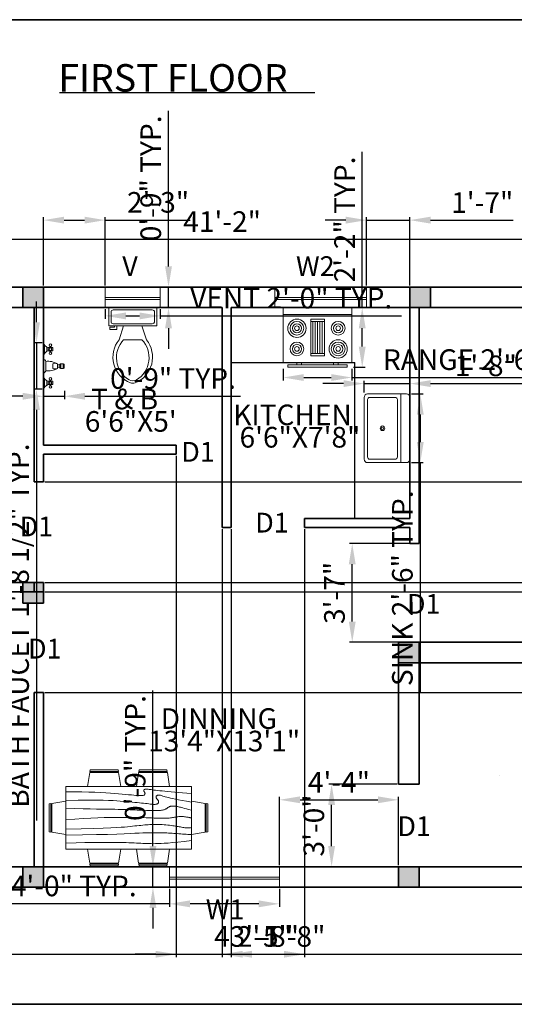
# Model space of a CAD drawing. Units: inches. Extents: x -281 to 2337, y 1647 to 2113.
# Tile 5 of 6: x 1906 to 2121, y 1674 to 2103. Entities that reach past the tile are written whole.
import ezdxf

# ---------------------------------------------------------------- set-up
doc = ezdxf.new("R2010")
doc.units = ezdxf.units.IN
for name, color, linetype, lineweight in [('A-ANNO-DIMS', 242, 'Continuous', 18), ('A-ANNO-IDEN', 11, 'Continuous', 18), ('A-ANNO-TEXT', 7, 'Continuous', 25), ('A-ANNO-TTLB', 7, 'Continuous', 35), ('A-AREA-IDEN', 7, 'Continuous', 18), ('A-COLS', 1, 'Continuous', 35), ('A-EQPM', 8, 'Continuous', 18), ('A-FLOR-CASE', 8, 'Continuous', 25), ('A-FLOR-FIXT', 8, 'Continuous', 18), ('A-FLOR-STRS', 7, 'Continuous', 18), ('A-FURN', 8, 'Continuous', 18), ('A-GLAZ', 3, 'Continuous', 18), ('A-WALL', 7, 'Continuous', 35)]:
    doc.layers.add(name, color=color, linetype=linetype, lineweight=lineweight)
doc.styles.get("Standard").update_dxf_attribs({"font": 'arial.ttf'})
doc.dimstyles.new('ISO-25', dxfattribs={"dimtxt": 9, "dimasz": 9, "dimexe": 1.25, "dimexo": 0.625, "dimgap": 2, "dimtad": 1, "dimdec": 1, "dimlunit": 4, "dimtxsty": 'Standard', "dimcen": 2.5, "dimadec": 0, "dimazin": 0, "dimtfac": 1, "dimtdec": 1, "dimtmove": 0, "dimatfit": 3, "dimfxl": 1, "dimarcsym": 0})

# ---------------------------------------------------------------- blocks, each defined once
blk = doc.blocks.new('Range-Oven - 30 in top')
for p, q in [((0, -3), (30, -3)), ((12, -6), (18, -6)), ((13, -20), (13, -6)), ((14, -6), (14, -20)), ((15, -20), (15, -6)), ((16, -6), (16, -20)), ((17, -20), (17, -6)), ((18, -20), (12, -20)), ((6, -24), (6, -25)), ((8, -25), (8, -24)), ((22, -25), (22, -24)), ((24, -24), (24, -25))]:
    blk.add_line(p, q)
for points in [[(0, -24), (0, 0), (30, 0), (30, -24)], [(12, -21), (12, -5), (18, -5), (18, -21)], [(2, -26), (2, -25), (28, -25), (28, -26)]]:
    blk.add_lwpolyline(points, close=True)
for centre, radius in [((6, -9), 4), ((6, -9), 3), ((6, -9), 2), ((6, -9), 1), ((24, -9), 3), ((24, -9), 2), ((24, -9), 1), ((6, -18), 3), ((6, -18), 2), ((6, -18), 1), ((24, -18), 4), ((24, -18), 3), ((24, -18), 2), ((24, -18), 1)]:
    blk.add_circle(centre, radius)
blk = doc.blocks.new('Sink-single - 30 in top')
blk.add_line((-15, -3.999996), (15, -3.999996))
for points in [[(-13.5, 0), (13.5, 0)], [(-15, -18.499996), (-15, -1.5)], [(15, -1.5), (15, -18.499996)], [(-13.5, -17.499996), (-13.5, -6.499996)], [(-12.5, -5.499996), (12.5, -5.499996)], [(13.5, -6.499996), (13.5, -17.499996)], [(13.5, -19.999996), (-13.5, -19.999996)], [(12.5, -18.499996), (-12.5, -18.499996)]]:
    blk.add_lwpolyline(points)
for radius in [1, 0.5]:
    blk.add_circle((0, -11.999996), radius)
for centre, radius, start, end in [((-13.5, -1.5), 1.5, 90, 180), ((13.5, -1.5), 1.5, 0, 90), ((-12.5, -6.499996), 1, 90, 180), ((12.5, -6.499996), 1, 0, 90), ((-13.5, -18.499996), 1.5, 180, 270), ((-12.5, -17.499996), 1, 180, 270), ((12.5, -17.499996), 1, 270, 0), ((13.5, -18.499996), 1.5, 270, 0)]:
    blk.add_arc(centre, radius, start, end)
blk = doc.blocks.new('Toilet - top')
for p, q in [((9.5, -6), (9.5, -2)), ((-10, -8.5), (-8, -8.5)), ((-10, -9.5), (-10, -8.5)), ((-8, -8.5), (-8, -8)), ((-7, -8), (-7, -9.5)), ((-4, -8), (-6, -14)), ((4, -8), (6, -14)), ((-7, -9.5), (-10, -9.5)), ((4, -14), (-4, -14))]:
    blk.add_line(p, q)
blk.add_lwpolyline([(10.5, -8), (10.5, 0), (-10.5, 0), (-10.5, -8)], close=True)
for points in [[(-9.5, -2), (-9.5, -6)], [(8.5, -1), (-8.5, -1)], [(-8.5, -7), (8.5, -7)]]:
    blk.add_lwpolyline(points)
for centre, radius, start, end in [((-8.62, -1.88), 0.884, 81.8699, 188.1301), ((8.62, -1.88), 0.884, 351.8699, 98.1301), ((-8.62, -6.12), 0.884, 171.8699, 278.1301), ((8.62, -6.12), 0.884, 261.8699, 8.1301), ((3.52, -21.58), 12.17, 141.4691, 247.9714), ((4.2, -21.82), 11.33, 136.3677, 238.9468), ((-3.52, -21.58), 12.17, 292.0284, 38.5307), ((-4.2, -21.82), 11.33, 301.053, 43.6321), ((0, -27.88), 4, 245.7318, 294.2682), ((0, -29), 4, 254.8605, 285.1395)]:
    blk.add_arc(centre, radius, start, end)
blk = doc.blocks.new('Faucet - Bathroom front')
for p, q in [((-0.5, 4.25), (0.5, 4.25)), ((0.5, 3.75), (-0.5, 3.75)), ((-0.5, 3), (0.5, 3)), ((-0.25, 3), (-0.25, 3.5)), ((0.25, 3.5), (0.25, 3)), ((-5, 0), (-2.25, 0)), ((-4.5087, 0.25), (-2.7408, 0.25)), ((-4, 1.625), (-4.25, 1.625)), ((-4, 1.375), (-4.25, 1.375)), ((-3.1442, 0.75), (-4.0979, 0.75)), ((-3.25, 1.625), (-3, 1.625)), ((-3.25, 1.375), (-3, 1.375)), ((-1.5, 0), (1.5, 0)), ((-1, 0.5), (1, 0.5)), ((0.5, 2), (-0.5, 2)), ((2.25, 0), (5, 0)), ((2.7413, 0.25), (4.5092, 0.25)), ((3.25, 1.625), (3, 1.625)), ((3.25, 1.375), (3, 1.375)), ((4.1058, 0.75), (3.1521, 0.75)), ((4, 1.625), (4.25, 1.625)), ((4, 1.375), (4.25, 1.375))]:
    blk.add_line(p, q)
for points in [[(-0.5, 3.75), (-0.5, 4.25)], [(-0.25, 4.5), (0.25, 4.5)], [(0.5, 4.25), (0.5, 3.75)], [(0.25, 3.5), (-0.25, 3.5)]]:
    blk.add_lwpolyline(points)
for points in [[(-4, 1), (-4, 2), (-3.25, 2), (-3.25, 1)], [(3.25, 1), (3.25, 2), (4, 2), (4, 1)]]:
    blk.add_lwpolyline(points, close=True)
for centre in [(-4.5, 1.5), (-3.625, 1.5), (-2.75, 1.5), (2.75, 1.5), (3.625, 1.5), (4.5, 1.5)]:
    blk.add_circle(centre, 0.2795)
for centre, radius, start, end in [((-0.2575, 4.2575), 0.2426, 88.22243, 181.7776), ((0.2575, 4.2575), 0.2426, 358.2224, 91.77757), ((3, 1), 4.0311, 150.2551, 187.125), ((0.6413, 2.5), 1.246, 156.3417, 203.6583), ((-0.2575, 3.7425), 0.2426, 178.2224, 271.7776), ((0.2575, 3.7425), 0.2426, 268.2224, 1.777565), ((-3, 1), 4.0311, 352.875, 29.74488), ((-0.6413, 2.5), 1.246, 336.3417, 23.65835), ((-5.375, 1.375), 1.4252, 285.2551, 344.7449), ((-1.875, 1.375), 1.4252, 195.2551, 254.7449), ((-0.7962, -0.2038), 0.7327, 106.1502, 163.8498), ((0.7962, -0.2038), 0.7327, 16.1502, 73.84979), ((1.875, 1.375), 1.4252, 285.2551, 344.7449), ((5.375, 1.375), 1.4252, 195.2551, 254.7449)]:
    blk.add_arc(centre, radius, start, end)
blk = doc.blocks.new('Dining Set - 36 x 72 in.')
for p, q in [((-22.2343, 26.00059), (-23.4847, 17.99762)), ((-22.2304, 26), (-5.7608, 26)), ((-22, 27.5), (-22.1562, 26.50042)), ((-5.8416, 26.5), (-22.1534, 26.5)), ((-22, 27.5), (-6, 27.5)), ((-5.8437, 26.49966), (-6, 27.5)), ((-4.5152, 17.99762), (-5.7655, 25.99926)), ((5.7657, 26.00059), (4.5153, 17.99762)), ((5.7696, 26), (22.2392, 26)), ((6, 27.5), (5.8438, 26.50042)), ((22.1584, 26.5), (5.8466, 26.5)), ((6, 27.5), (22, 27.5)), ((22.1563, 26.49966), (22, 27.5)), ((23.4848, 17.99762), (22.2345, 25.99926)), ((36, 18), (-36, 18)), ((-36, 18), (-36, -18)), ((36, -18), (36, 18)), ((-45.5, 8), (-44.5004, 8.15617)), ((-45.5, 8), (-45.5, -8)), ((-44.5, -8.15843), (-44.5, 8.15338)), ((-44.0006, 8.23428), (-35.9976, 9.48474)), ((-44, 8.23041), (-44, -8.23915)), ((44.0006, 8.23428), (35.9976, 9.48474)), ((44, 8.23041), (44, -8.23915)), ((44.5, -8.15843), (44.5, 8.15338)), ((45.5, 8), (44.5005, 8.15617)), ((45.5, 8), (45.5, -8)), ((-44.4997, -8.15631), (-45.5, -8)), ((-35.9976, -9.48476), (-43.9993, -8.2345)), ((35.9976, -9.48476), (43.9993, -8.2345)), ((44.4997, -8.15631), (45.5, -8)), ((-36, -18), (36, -18)), ((-22.2343, -26.0006), (-23.4847, -17.99762)), ((-4.5152, -17.99762), (-5.7655, -25.99928)), ((5.7657, -26.0006), (4.5153, -17.99762)), ((23.4848, -17.99762), (22.2345, -25.99928)), ((-22.2304, -26), (-5.7608, -26)), ((-22, -27.5), (-22.1562, -26.50044)), ((-5.8416, -26.5), (-22.1534, -26.5)), ((-22, -27.5), (-6, -27.5)), ((-5.8437, -26.49967), (-6, -27.5)), ((5.7696, -26), (22.2392, -26)), ((6, -27.5), (5.8438, -26.50044)), ((22.1584, -26.5), (5.8466, -26.5)), ((6, -27.5), (22, -27.5)), ((22.1563, -26.49967), (22, -27.5))]:
    blk.add_line(p, q)
for points in [[(-36, 15), (-31.1772, 14.97754), (-26.8079, 14.91406), (-22.8538, 14.81543), (-19.276, 14.6875), (-16.0362, 14.53613), (-13.0957, 14.36718), (-10.4159, 14.18652), (-7.9583, 14), (-5.6904, 13.81315), (-3.6035, 13.63021), (-1.6954, 13.45508), (0.0365, 13.29166), (1.5945, 13.14388), (2.9811, 13.01562), (4.1988, 12.9108), (5.25, 12.83333), (6.1393, 12.78613), (6.8802, 12.76823), (7.4883, 12.77767), (7.9792, 12.8125), (8.3685, 12.87077), (8.6719, 12.95052), (8.9049, 13.0498), (9.0833, 13.16666), (9.2205, 13.29899), (9.3216, 13.44401), (9.3895, 13.59879), (9.4271, 13.76041), (9.4373, 13.92594), (9.4232, 14.09245), (9.3875, 14.257), (9.3333, 14.41666), (9.2638, 14.56917), (9.1836, 14.71484), (9.0975, 14.85465), (9.0104, 14.98958), (8.9272, 15.1206), (8.8529, 15.2487), (8.7922, 15.37483), (8.75, 15.5), (8.7305, 15.62467), (8.7344, 15.74739), (8.7617, 15.86621), (8.8125, 15.97916), (8.8867, 16.08431), (8.9844, 16.17968), (9.1055, 16.26334), (9.25, 16.33333), (9.4189, 16.38802), (9.6172, 16.42708), (9.8506, 16.45052), (10.125, 16.45833), (10.4463, 16.45052), (10.8203, 16.42708), (11.2529, 16.38802), (11.75, 16.33333), (12.3184, 16.26318), (12.9694, 16.17838), (13.7151, 16.07991), (14.5677, 15.96875), (15.5395, 15.84586), (16.6426, 15.71224), (17.8893, 15.56884), (19.2917, 15.41666), (20.859, 15.25667), (22.5879, 15.08984), (24.4721, 14.91715), (26.5052, 14.73958), (28.6809, 14.5581), (30.9929, 14.3737), (33.4347, 14.18733), (36, 14)], [(-36, 10), (-28.9766, 10.14274), (-23.1725, 10.20442), (-18.4241, 10.19775), (-14.5677, 10.13541), (-11.4399, 10.03011), (-8.877, 9.89453), (-6.7154, 9.74137), (-4.7917, 9.58333), (-2.9698, 9.43082), (-1.2246, 9.28515), (0.4415, 9.14534), (2.026, 9.01041), (3.5266, 8.87939), (4.9408, 8.7513), (6.266, 8.62516), (7.5, 8.5), (8.6411, 8.37549), (9.6914, 8.2539), (10.6538, 8.13818), (11.5312, 8.03125), (12.3267, 7.93603), (13.043, 7.85547), (13.6831, 7.79248), (14.25, 7.75), (14.7471, 7.7303), (15.1797, 7.73307), (15.5537, 7.75732), (15.875, 7.80208), (16.1494, 7.86637), (16.3828, 7.94922), (16.5811, 8.04964), (16.75, 8.16666), (16.8944, 8.29915), (17.0143, 8.44531), (17.1089, 8.60319), (17.1771, 8.77083), (17.218, 8.94629), (17.2305, 9.1276), (17.2137, 9.31282), (17.1667, 9.5), (17.0895, 9.6875), (16.987, 9.875), (16.8649, 10.0625), (16.7292, 10.25), (16.5856, 10.4375), (16.4401, 10.625), (16.2985, 10.8125), (16.1667, 11), (16.05, 11.18733), (15.9518, 11.3737), (15.8752, 11.5581), (15.8229, 11.73958), (15.798, 11.91715), (15.8034, 12.08984), (15.842, 12.25667), (15.9167, 12.41666), (16.0295, 12.56836), (16.1784, 12.70833), (16.3605, 12.83268), (16.5729, 12.9375), (16.8127, 13.01888), (17.0768, 13.07291), (17.3625, 13.0957), (17.6667, 13.08333), (17.9894, 13.03312), (18.3418, 12.94726), (18.7382, 12.82918), (19.1927, 12.68229), (19.7195, 12.51001), (20.3327, 12.31575), (21.0465, 12.10294), (21.875, 11.875), (22.8357, 11.63354), (23.959, 11.37304), (25.2786, 11.08618), (26.8282, 10.76562), (28.6414, 10.40405), (30.752, 9.99414), (33.1936, 9.52856), (36, 9)], [(-36, 5.5), (-30.7157, 5.3348), (-26.069, 5.20963), (-21.9946, 5.11767), (-18.4271, 5.05208), (-15.3009, 5.00602), (-12.5508, 4.97265), (-10.1112, 4.94515), (-7.9167, 4.91666), (-5.909, 4.88167), (-4.0586, 4.83984), (-2.3429, 4.79215), (-0.7396, 4.73958), (0.7739, 4.6831), (2.22, 4.6237), (3.6213, 4.56233), (5, 4.5), (6.373, 4.43782), (7.7344, 4.3776), (9.0723, 4.32129), (10.375, 4.27083), (11.6309, 4.22819), (12.8281, 4.19531), (13.9551, 4.17415), (15, 4.16666), (15.954, 4.17448), (16.819, 4.19791), (17.6001, 4.23698), (18.3021, 4.29166), (18.9299, 4.36198), (19.4883, 4.44791), (19.9823, 4.54948), (20.4167, 4.66666), (20.7969, 4.79899), (21.1302, 4.94401), (21.4245, 5.09879), (21.6875, 5.26041), (21.9271, 5.42594), (22.1511, 5.59245), (22.3672, 5.757), (22.5834, 5.91666), (22.8065, 6.06868), (23.0404, 6.21093), (23.2879, 6.34147), (23.5521, 6.45833), (23.8358, 6.55957), (24.142, 6.64323), (24.4735, 6.70735), (24.8334, 6.75), (25.2235, 6.76969), (25.642, 6.76692), (26.0858, 6.74267), (26.5521, 6.69791), (27.0379, 6.63362), (27.5404, 6.55078), (28.0565, 6.45036), (28.5834, 6.33333), (29.1242, 6.19987), (29.7071, 6.04687), (30.3661, 5.87044), (31.1354, 5.66666), (32.0493, 5.43164), (33.142, 5.16146), (34.4475, 4.85221), (36, 4.5)], [(-36, -1), (-30.7915, -0.6591), (-26.0195, -0.38216), (-21.6519, -0.16284), (-17.6563, 0.00521), (-14.0005, 0.12833), (-10.6523, 0.21289), (-7.5796, 0.26522), (-4.75, 0.29166), (-2.134, 0.29793), (0.2878, 0.28711), (2.5317, 0.26163), (4.6146, 0.22396), (6.5529, 0.17651), (8.3633, 0.12174), (10.0623, 0.06209), (11.6667, 0), (13.1899, -0.06201), (14.6341, -0.1211), (15.9982, -0.17432), (17.2813, -0.21875), (18.4823, -0.25147), (19.6003, -0.26953), (20.6343, -0.27002), (21.5834, -0.25), (22.4481, -0.20768), (23.2357, -0.14584), (23.9549, -0.06836), (24.6146, 0.02083), (25.2235, 0.11784), (25.7904, 0.21875), (26.3241, 0.31966), (26.8334, 0.41666), (27.3265, 0.50618), (27.8099, 0.58593), (28.2894, 0.65397), (28.7709, 0.70833), (29.2601, 0.74707), (29.763, 0.76823), (30.2855, 0.76985), (30.8334, 0.75), (31.4088, 0.70784), (31.9994, 0.64713), (32.589, 0.57275), (33.1615, 0.48958), (33.7008, 0.4025), (34.1908, 0.3164), (34.6153, 0.23616), (34.9584, 0.16666), (35.2099, 0.11165), (35.3848, 0.07031), (35.504, 0.04069), (35.5886, 0.02083), (35.6594, 0.00879), (35.7377, 0.0026), (35.8442, 0.00032), (36, 0)], [(-36, -6.5), (-27.1843, -6.31267), (-20.084, -6.1263), (-14.469, -5.9419), (-10.1094, -5.76042), (-6.7752, -5.58285), (-4.2363, -5.41016), (-2.2629, -5.24333), (-0.625, -5.08334), (0.8708, -4.93099), (2.2715, -4.78646), (3.5872, -4.64974), (4.8281, -4.52084), (6.0046, -4.39974), (7.127, -4.28646), (8.2053, -4.18099), (9.25, -4.08334), (10.2705, -3.99382), (11.2734, -3.91407), (12.2647, -3.84603), (13.25, -3.79167), (14.2354, -3.75293), (15.2266, -3.73177), (16.2295, -3.73015), (17.25, -3.75), (18.2912, -3.79248), (19.3451, -3.85547), (20.4009, -3.93604), (21.4479, -4.03125), (22.4754, -4.13819), (23.4727, -4.25391), (24.4289, -4.37549), (25.3334, -4.5), (26.1785, -4.62492), (26.9694, -4.74935), (27.7145, -4.87281), (28.4219, -4.99479), (29.1, -5.11483), (29.7572, -5.23242), (30.4016, -5.34709), (31.0417, -5.45834), (31.6837, -5.56437), (32.3262, -5.65821), (32.9658, -5.73153), (33.599, -5.77604), (34.2224, -5.78345), (34.8327, -5.74545), (35.4264, -5.65373), (36, -5.5)], [(-36, -10), (-26.4022, -9.81299), (-18.4675, -9.62891), (-11.9839, -9.45069), (-6.7396, -9.28125), (-2.5226, -9.12354), (0.8789, -8.98047), (3.6769, -8.85498), (6.0833, -8.75), (8.2767, -8.66765), (10.3021, -8.60677), (12.1712, -8.56543), (13.8958, -8.54167), (15.4876, -8.53353), (16.9583, -8.53907), (18.3197, -8.55632), (19.5834, -8.58334), (20.7616, -8.61841), (21.8685, -8.66081), (22.9188, -8.71004), (23.9271, -8.76563), (24.9081, -8.82707), (25.8763, -8.89388), (26.8465, -8.96558), (27.8334, -9.04167), (28.8474, -9.12118), (29.8828, -9.20117), (30.93, -9.27824), (31.9792, -9.34896), (33.0205, -9.40991), (34.0443, -9.45768), (35.0407, -9.48885), (36, -9.5)], [(-36, -14.5), (-30.0881, -14.33513), (-25.0332, -14.21224), (-20.7312, -14.12647), (-17.0781, -14.07292), (-13.97, -14.04671), (-11.3027, -14.04297), (-8.9724, -14.05681), (-6.875, -14.08334), (-4.9224, -14.11833), (-3.0905, -14.16016), (-1.3709, -14.20785), (0.2448, -14.26042), (1.7647, -14.3169), (3.1973, -14.3763), (4.5507, -14.43767), (5.8333, -14.5), (7.0554, -14.5621), (8.235, -14.62175), (9.3922, -14.67652), (10.5469, -14.72396), (11.7192, -14.76164), (12.929, -14.78711), (14.1965, -14.79794), (15.5417, -14.79167), (16.9933, -14.76424), (18.6152, -14.70508), (20.4804, -14.60197), (22.6615, -14.44271), (25.2312, -14.21509), (28.2624, -13.9069), (31.8277, -13.50594), (36, -13)]]:
    blk.add_lwpolyline(points)
blk = doc.blocks.new('*D10')
at = {"layer": 'A-ANNO-DIMS', "color": 0, "lineweight": -2, "transparency": 16777216}
for p, q in [((1746.88, 1987.41), (1746.88, 2008.91)), ((1755.88, 2007.66), (2231.88, 2007.66)), ((2240.88, 1987.41), (2240.88, 2008.91))]:
    blk.add_line(p, q, dxfattribs=at)
at = {"layer": 'A-ANNO-DIMS', "color": 0, "transparency": 16777216}
for points in [[(1755.88, 2009.16), (1755.88, 2006.16), (1746.88, 2007.66)], [(2231.88, 2009.16), (2231.88, 2006.16), (2240.88, 2007.66)]]:
    blk.add_solid(points, dxfattribs=at)
at = {"layer": 'Defpoints', "color": 0, "transparency": 16777216}
for p in [(2240.88, 2007.66), (1746.88, 1986.79), (2240.88, 1986.79)]:
    blk.add_point(p, dxfattribs=at)
at = {"layer": 'A-ANNO-DIMS', "color": 0, "transparency": 16777216, "insert": (1993.88, 2014.18), "char_height": 9, "attachment_point": 5}
blk.add_mtext('41\'-2"', dxfattribs=at)
blk = doc.blocks.new('COL-9x9')
h = blk.add_hatch(color=256)
h.dxf.hatch_style = 1
h.paths.add_polyline_path([(9, 9), (0, 9), (0, 0), (9, 0)])
for p, q in [((0, 9), (9, 9)), ((0, 0), (0, 9)), ((9, 9), (9, 0)), ((9, 0), (0, 0))]:
    blk.add_line(p, q)
blk = doc.blocks.new('WIN-W1-48')
for p, q in [((0, 48), (9, 48)), ((3.5, 0), (3.5, 48)), ((4.5, 0), (4.5, 48)), ((0, 0), (9, 0))]:
    blk.add_line(p, q)
blk = doc.blocks.new('WIN-W2-40')
for p, q in [((0, 0), (0, 9)), ((40, 0), (40, 9)), ((0, 4.5), (40, 4.5)), ((0, 3.5), (40, 3.5))]:
    blk.add_line(p, q)
blk = doc.blocks.new('VENT-24')
for p, q in [((0, 0), (0, 9)), ((24, 0), (24, 9)), ((0, 4.5), (24, 4.5)), ((0, 3.5), (24, 3.5))]:
    blk.add_line(p, q)
blk = doc.blocks.new('COUNTER-L')
for p in [(0, 68), (54, 0)]:
    blk.add_line(p, (54, 68))
blk = doc.blocks.new('*D19')
at = {"layer": 'A-ANNO-DIMS', "color": 0, "lineweight": -2, "transparency": 16777216}
for p, q in [((1970.88, 1724.16), (1970.88, 1716.34)), ((2018.88, 1724.16), (2018.88, 1716.34)), ((1970.88, 1717.59), (1821.64, 1717.59)), ((2009.88, 1717.59), (1979.88, 1717.59))]:
    blk.add_line(p, q, dxfattribs=at)
at = {"layer": 'A-ANNO-DIMS', "color": 0, "transparency": 16777216}
for points in [[(1979.88, 1719.09), (1979.88, 1716.09), (1970.88, 1717.59)], [(2009.88, 1719.09), (2009.88, 1716.09), (2018.88, 1717.59)]]:
    blk.add_solid(points, dxfattribs=at)
at = {"layer": 'Defpoints', "color": 0, "transparency": 16777216}
for p in [(1970.88, 1724.79), (2018.88, 1724.79), (1970.88, 1717.59)]:
    blk.add_point(p, dxfattribs=at)
at = {"layer": 'A-ANNO-DIMS', "color": 0, "transparency": 16777216, "insert": (1891.76, 1724.24), "char_height": 9, "attachment_point": 5}
blk.add_mtext('WINDOW W1 4\'-0" TYP.', dxfattribs=at)
blk = doc.blocks.new('*D20')
at = {"layer": 'A-ANNO-DIMS', "color": 0, "lineweight": -2, "transparency": 16777216}
for p, q in [((1963.68, 1742.79), (1963.68, 1810.65)), ((1970.26, 1733.79), (1962.43, 1733.79)), ((1963.68, 1724.79), (1963.68, 1733.79)), ((1970.26, 1724.79), (1962.43, 1724.79)), ((1963.68, 1715.79), (1963.68, 1706.79))]:
    blk.add_line(p, q, dxfattribs=at)
at = {"layer": 'A-ANNO-DIMS', "color": 0, "transparency": 16777216}
for points in [[(1962.18, 1742.79), (1965.18, 1742.79), (1963.68, 1733.79)], [(1962.18, 1715.79), (1965.18, 1715.79), (1963.68, 1724.79)]]:
    blk.add_solid(points, dxfattribs=at)
at = {"layer": 'Defpoints', "color": 0, "transparency": 16777216}
for p in [(1963.68, 1733.79), (1970.88, 1733.79), (1970.88, 1724.79)]:
    blk.add_point(p, dxfattribs=at)
at = {"layer": 'A-ANNO-DIMS', "color": 0, "transparency": 16777216, "insert": (1957.09, 1781.22), "char_height": 9, "attachment_point": 5, "rotation": 90}
blk.add_mtext('0\'-9" TYP.', dxfattribs=at)
blk = doc.blocks.new('*D23')
at = {"layer": 'A-ANNO-DIMS', "color": 0, "lineweight": -2, "transparency": 16777216}
for p, q in [((1942.88, 1977.16), (1942.88, 1972.94)), ((1966.88, 1977.16), (1966.88, 1972.94)), ((1951.88, 1974.19), (1957.88, 1974.19)), ((1966.88, 1974.19), (2072.23, 1974.19))]:
    blk.add_line(p, q, dxfattribs=at)
at = {"layer": 'A-ANNO-DIMS', "color": 0, "transparency": 16777216}
for points in [[(1951.88, 1975.69), (1951.88, 1972.69), (1942.88, 1974.19)], [(1957.88, 1975.69), (1957.88, 1972.69), (1966.88, 1974.19)]]:
    blk.add_solid(points, dxfattribs=at)
at = {"layer": 'Defpoints', "color": 0, "transparency": 16777216}
for p in [(1942.88, 1977.79), (1966.88, 1977.79), (1966.88, 1974.19)]:
    blk.add_point(p, dxfattribs=at)
at = {"layer": 'A-ANNO-DIMS', "color": 0, "transparency": 16777216, "insert": (2024.06, 1980.78), "char_height": 9, "attachment_point": 5}
blk.add_mtext('VENT 2\'-0" TYP.', dxfattribs=at)
blk = doc.blocks.new('*D24')
at = {"layer": 'A-ANNO-DIMS', "color": 0, "lineweight": -2, "transparency": 16777216}
for p, q in [((1970.48, 1995.79), (1970.48, 2063.65)), ((1967.51, 1986.79), (1971.73, 1986.79)), ((1970.48, 1977.79), (1970.48, 1986.79)), ((1967.51, 1977.79), (1971.73, 1977.79)), ((1970.48, 1968.79), (1970.48, 1959.79))]:
    blk.add_line(p, q, dxfattribs=at)
at = {"layer": 'A-ANNO-DIMS', "color": 0, "transparency": 16777216}
for points in [[(1968.98, 1995.79), (1971.98, 1995.79), (1970.48, 1986.79)], [(1968.98, 1968.79), (1971.98, 1968.79), (1970.48, 1977.79)]]:
    blk.add_solid(points, dxfattribs=at)
at = {"layer": 'Defpoints', "color": 0, "transparency": 16777216}
for p in [(1966.88, 1986.79), (1970.48, 1986.79), (1966.88, 1977.79)]:
    blk.add_point(p, dxfattribs=at)
at = {"layer": 'A-ANNO-DIMS', "color": 0, "transparency": 16777216, "insert": (1963.89, 2034.22), "char_height": 9, "attachment_point": 5, "rotation": 90}
blk.add_mtext('0\'-9" TYP.', dxfattribs=at)
blk = doc.blocks.new('*D31')
at = {"layer": 'A-ANNO-DIMS', "color": 0, "lineweight": -2, "transparency": 16777216}
for p, q in [((2020.54, 1951.16), (2020.54, 1946.04)), ((2050.54, 1951.16), (2050.54, 1946.04)), ((2029.54, 1947.29), (2041.54, 1947.29)), ((2050.54, 1947.29), (2166.14, 1947.29))]:
    blk.add_line(p, q, dxfattribs=at)
at = {"layer": 'A-ANNO-DIMS', "color": 0, "transparency": 16777216}
for points in [[(2029.54, 1948.79), (2029.54, 1945.79), (2020.54, 1947.29)], [(2041.54, 1948.79), (2041.54, 1945.79), (2050.54, 1947.29)]]:
    blk.add_solid(points, dxfattribs=at)
at = {"layer": 'Defpoints', "color": 0, "transparency": 16777216}
for p in [(2020.54, 1951.79), (2050.54, 1951.79), (2050.54, 1947.29)]:
    blk.add_point(p, dxfattribs=at)
at = {"layer": 'A-ANNO-DIMS', "color": 0, "transparency": 16777216, "insert": (2112.84, 1953.94), "char_height": 9, "attachment_point": 5}
blk.add_mtext('RANGE 2\'-6" TYP.', dxfattribs=at)
blk = doc.blocks.new('*D32')
at = {"layer": 'A-ANNO-DIMS', "color": 0, "lineweight": -2, "transparency": 16777216}
for p, q in [((2055.04, 1977.79), (2055.04, 2045.8)), ((2051.17, 1977.79), (2056.29, 1977.79)), ((2055.04, 1960.79), (2055.04, 1968.79)), ((2051.17, 1951.79), (2056.29, 1951.79))]:
    blk.add_line(p, q, dxfattribs=at)
at = {"layer": 'A-ANNO-DIMS', "color": 0, "transparency": 16777216}
for points in [[(2053.54, 1968.79), (2056.54, 1968.79), (2055.04, 1977.79)], [(2053.54, 1960.79), (2056.54, 1960.79), (2055.04, 1951.79)]]:
    blk.add_solid(points, dxfattribs=at)
at = {"layer": 'Defpoints', "color": 0, "transparency": 16777216}
for p in [(2050.54, 1977.79), (2055.04, 1977.79), (2050.54, 1951.79)]:
    blk.add_point(p, dxfattribs=at)
at = {"layer": 'A-ANNO-DIMS', "color": 0, "transparency": 16777216, "insert": (2048.52, 2016.29), "char_height": 9, "attachment_point": 5, "rotation": 90}
blk.add_mtext('2\'-2" TYP.', dxfattribs=at)
blk = doc.blocks.new('*D33')
at = {"layer": 'A-ANNO-DIMS', "color": 0, "lineweight": -2, "transparency": 16777216}
for p, q in [((2076.51, 1940.14), (2081.63, 1940.14)), ((2080.38, 1931.14), (2080.38, 1919.14)), ((2076.51, 1910.14), (2081.63, 1910.14)), ((2080.38, 1910.14), (2080.38, 1809.49))]:
    blk.add_line(p, q, dxfattribs=at)
at = {"layer": 'A-ANNO-DIMS', "color": 0, "transparency": 16777216}
for points in [[(2078.88, 1931.14), (2081.88, 1931.14), (2080.38, 1940.14)], [(2078.88, 1919.14), (2081.88, 1919.14), (2080.38, 1910.14)]]:
    blk.add_solid(points, dxfattribs=at)
at = {"layer": 'Defpoints', "color": 0, "transparency": 16777216}
for p in [(2075.88, 1940.14), (2075.88, 1910.14), (2080.38, 1910.14)]:
    blk.add_point(p, dxfattribs=at)
at = {"layer": 'A-ANNO-DIMS', "color": 0, "transparency": 16777216, "insert": (2073.73, 1855.32), "char_height": 9, "attachment_point": 5, "rotation": 90}
blk.add_mtext('SINK 2\'-6" TYP.', dxfattribs=at)
blk = doc.blocks.new('*D34')
at = {"layer": 'A-ANNO-DIMS', "color": 0, "lineweight": -2, "transparency": 16777216}
for p, q in [((2046.88, 1944.64), (2037.88, 1944.64)), ((2055.88, 1940.77), (2055.88, 1945.89)), ((2055.88, 1944.64), (2075.88, 1944.64)), ((2075.88, 1940.77), (2075.88, 1945.89)), ((2084.88, 1944.64), (2151.89, 1944.64))]:
    blk.add_line(p, q, dxfattribs=at)
at = {"layer": 'A-ANNO-DIMS', "color": 0, "transparency": 16777216}
for points in [[(2046.88, 1946.14), (2046.88, 1943.14), (2055.88, 1944.64)], [(2084.88, 1946.14), (2084.88, 1943.14), (2075.88, 1944.64)]]:
    blk.add_solid(points, dxfattribs=at)
at = {"layer": 'Defpoints', "color": 0, "transparency": 16777216}
for p in [(2075.88, 1944.64), (2055.88, 1940.14), (2075.88, 1940.14)]:
    blk.add_point(p, dxfattribs=at)
at = {"layer": 'A-ANNO-DIMS', "color": 0, "transparency": 16777216, "insert": (2122.89, 1951.24), "char_height": 9, "attachment_point": 5}
blk.add_mtext('1\'-8" TYP.', dxfattribs=at)
blk = doc.blocks.new('*D39')
at = {"layer": 'A-ANNO-DIMS', "color": 0, "lineweight": -2, "transparency": 16777216}
for p, q in [((1912.84, 1971.43), (1912.84, 1980.43)), ((1915.26, 1962.43), (1911.59, 1962.43)), ((1912.84, 1962.43), (1912.84, 1942.15)), ((1915.26, 1942.15), (1911.59, 1942.15)), ((1912.84, 1933.15), (1912.84, 1753.91))]:
    blk.add_line(p, q, dxfattribs=at)
at = {"layer": 'A-ANNO-DIMS', "color": 0, "transparency": 16777216}
for points in [[(1911.34, 1971.43), (1914.34, 1971.43), (1912.84, 1962.43)], [(1911.34, 1933.15), (1914.34, 1933.15), (1912.84, 1942.15)]]:
    blk.add_solid(points, dxfattribs=at)
at = {"layer": 'Defpoints', "color": 0, "transparency": 16777216}
for p in [(1915.88, 1962.43), (1912.84, 1942.15), (1915.88, 1942.15)]:
    blk.add_point(p, dxfattribs=at)
at = {"layer": 'A-ANNO-DIMS', "color": 0, "transparency": 16777216, "insert": (1906.19, 1839.03), "char_height": 9, "attachment_point": 5, "rotation": 90}
blk.add_mtext('BATH FAUCET 1\'-8 1/2" TYP.', dxfattribs=at)
blk = doc.blocks.new('*D40')
at = {"layer": 'A-ANNO-DIMS', "color": 0, "lineweight": -2, "transparency": 16777216}
for p, q in [((1906.88, 1939.11), (1897.88, 1939.11)), ((1915.88, 1941.53), (1915.88, 1937.86)), ((1915.88, 1939.11), (1925.01, 1939.11)), ((1925.01, 1941.53), (1925.01, 1937.86)), ((1934.01, 1939.11), (2001.87, 1939.11))]:
    blk.add_line(p, q, dxfattribs=at)
at = {"layer": 'A-ANNO-DIMS', "color": 0, "transparency": 16777216}
for points in [[(1906.88, 1940.61), (1906.88, 1937.61), (1915.88, 1939.11)], [(1934.01, 1940.61), (1934.01, 1937.61), (1925.01, 1939.11)]]:
    blk.add_solid(points, dxfattribs=at)
at = {"layer": 'Defpoints', "color": 0, "transparency": 16777216}
for p in [(1915.88, 1942.15), (1925.01, 1942.15), (1925.01, 1939.11)]:
    blk.add_point(p, dxfattribs=at)
at = {"layer": 'A-ANNO-DIMS', "color": 0, "transparency": 16777216, "insert": (1972.44, 1945.7), "char_height": 9, "attachment_point": 5}
blk.add_mtext('0\'-9" TYP.', dxfattribs=at)
blk = doc.blocks.new('*D41')
at = {"layer": 'A-ANNO-DIMS', "color": 0, "lineweight": -2, "transparency": 16777216}
for p, q in [((1746.88, 1724.16), (1746.88, 1694.33)), ((2267.88, 1724.16), (2267.88, 1694.33)), ((1755.88, 1695.58), (2258.88, 1695.58))]:
    blk.add_line(p, q, dxfattribs=at)
at = {"layer": 'A-ANNO-DIMS', "color": 0, "transparency": 16777216}
for points in [[(1755.88, 1697.08), (1755.88, 1694.08), (1746.88, 1695.58)], [(2258.88, 1697.08), (2258.88, 1694.08), (2267.88, 1695.58)]]:
    blk.add_solid(points, dxfattribs=at)
at = {"layer": 'Defpoints', "color": 0, "transparency": 16777216}
for p in [(1746.88, 1724.79), (2267.88, 1724.79), (2267.88, 1695.58)]:
    blk.add_point(p, dxfattribs=at)
at = {"layer": 'A-ANNO-DIMS', "color": 0, "transparency": 16777216, "insert": (2007.38, 1702.18), "char_height": 9, "attachment_point": 5}
blk.add_mtext('43\'-5"', dxfattribs=at)
blk = doc.blocks.new('*D51')
at = {"layer": 'A-ANNO-DIMS', "color": 0, "lineweight": -2, "transparency": 16777216}
for p, q in [((1997.88, 1881.16), (1997.88, 1694.33)), ((2029.88, 1881.16), (2029.88, 1694.33)), ((2006.88, 1695.58), (2020.88, 1695.58))]:
    blk.add_line(p, q, dxfattribs=at)
at = {"layer": 'A-ANNO-DIMS', "color": 0, "transparency": 16777216}
for points in [[(2006.88, 1697.08), (2006.88, 1694.08), (1997.88, 1695.58)], [(2020.88, 1697.08), (2020.88, 1694.08), (2029.88, 1695.58)]]:
    blk.add_solid(points, dxfattribs=at)
at = {"layer": 'Defpoints', "color": 0, "transparency": 16777216}
for p in [(1997.88, 1881.79), (2029.88, 1881.79), (2029.88, 1695.58)]:
    blk.add_point(p, dxfattribs=at)
at = {"layer": 'A-ANNO-DIMS', "color": 0, "transparency": 16777216, "insert": (2013.88, 1702.17), "char_height": 9, "attachment_point": 5}
blk.add_mtext('2\'-8"', dxfattribs=at)
blk = doc.blocks.new('*D52')
at = {"layer": 'A-ANNO-DIMS', "color": 0, "lineweight": -2, "transparency": 16777216}
for p, q in [((1973.88, 1913.16), (1973.88, 1694.33)), ((1993.88, 1881.16), (1993.88, 1694.33)), ((1964.88, 1695.58), (1955.88, 1695.58)), ((1973.88, 1695.58), (1993.88, 1695.58)), ((2002.88, 1695.58), (2038.96, 1695.58))]:
    blk.add_line(p, q, dxfattribs=at)
at = {"layer": 'A-ANNO-DIMS', "color": 0, "transparency": 16777216}
for points in [[(1964.88, 1697.08), (1964.88, 1694.08), (1973.88, 1695.58)], [(2002.88, 1697.08), (2002.88, 1694.08), (1993.88, 1695.58)]]:
    blk.add_solid(points, dxfattribs=at)
at = {"layer": 'Defpoints', "color": 0, "transparency": 16777216}
for p in [(1973.88, 1913.79), (1993.88, 1881.79), (1993.88, 1695.58)]:
    blk.add_point(p, dxfattribs=at)
at = {"layer": 'A-ANNO-DIMS', "color": 0, "transparency": 16777216, "insert": (2025.42, 1702.17), "char_height": 9, "attachment_point": 5}
blk.add_mtext('1\'-8"', dxfattribs=at)
blk = doc.blocks.new('*D53')
at = {"layer": 'A-ANNO-DIMS', "color": 0, "lineweight": -2, "transparency": 16777216}
for p, q in [((2070.26, 1769.79), (2040.43, 1769.79)), ((2041.68, 1742.79), (2041.68, 1760.79)), ((2070.26, 1733.79), (2040.43, 1733.79))]:
    blk.add_line(p, q, dxfattribs=at)
at = {"layer": 'A-ANNO-DIMS', "color": 0, "transparency": 16777216}
for points in [[(2040.18, 1760.79), (2043.18, 1760.79), (2041.68, 1769.79)], [(2040.18, 1742.79), (2043.18, 1742.79), (2041.68, 1733.79)]]:
    blk.add_solid(points, dxfattribs=at)
at = {"layer": 'Defpoints', "color": 0, "transparency": 16777216}
for p in [(2041.68, 1769.79), (2070.88, 1769.79), (2070.88, 1733.79)]:
    blk.add_point(p, dxfattribs=at)
at = {"layer": 'A-ANNO-DIMS', "color": 0, "transparency": 16777216, "insert": (2035.08, 1751.79), "char_height": 9, "attachment_point": 5, "rotation": 90}
blk.add_mtext('3\'-0"', dxfattribs=at)
blk = doc.blocks.new('*D54')
at = {"layer": 'A-ANNO-DIMS', "color": 0, "lineweight": -2, "transparency": 16777216}
for p, q in [((1916.51, 1901.79), (2298.33, 1901.79)), ((2297.08, 1866.79), (2297.08, 1892.79)), ((1916.51, 1857.79), (2298.33, 1857.79))]:
    blk.add_line(p, q, dxfattribs=at)
at = {"layer": 'A-ANNO-DIMS', "color": 0, "transparency": 16777216}
for points in [[(2295.58, 1892.79), (2298.58, 1892.79), (2297.08, 1901.79)], [(2295.58, 1866.79), (2298.58, 1866.79), (2297.08, 1857.79)]]:
    blk.add_solid(points, dxfattribs=at)
at = {"layer": 'Defpoints', "color": 0, "transparency": 16777216}
for p in [(1915.88, 1901.79), (2297.08, 1901.79), (1915.88, 1857.79)]:
    blk.add_point(p, dxfattribs=at)
at = {"layer": 'A-ANNO-DIMS', "color": 0, "transparency": 16777216, "insert": (2290.48, 1879.79), "char_height": 9, "attachment_point": 5, "rotation": 90}
blk.add_mtext('3\'-8"', dxfattribs=at)
blk = doc.blocks.new('*D55')
at = {"layer": 'A-ANNO-DIMS', "color": 0, "lineweight": -2, "transparency": 16777216}
for p, q in [((1916.51, 1853.79), (2298.33, 1853.79)), ((2297.08, 1818.79), (2297.08, 1844.79)), ((1916.51, 1809.79), (2298.33, 1809.79))]:
    blk.add_line(p, q, dxfattribs=at)
at = {"layer": 'A-ANNO-DIMS', "color": 0, "transparency": 16777216}
for points in [[(2295.58, 1844.79), (2298.58, 1844.79), (2297.08, 1853.79)], [(2295.58, 1818.79), (2298.58, 1818.79), (2297.08, 1809.79)]]:
    blk.add_solid(points, dxfattribs=at)
at = {"layer": 'Defpoints', "color": 0, "transparency": 16777216}
for p in [(1915.88, 1853.79), (2297.08, 1853.79), (1915.88, 1809.79)]:
    blk.add_point(p, dxfattribs=at)
at = {"layer": 'A-ANNO-DIMS', "color": 0, "transparency": 16777216, "insert": (2290.48, 1831.79), "char_height": 9, "attachment_point": 5, "rotation": 90}
blk.add_mtext('3\'-8"', dxfattribs=at)
blk = doc.blocks.new('*D56')
at = {"layer": 'A-ANNO-DIMS', "color": 0, "lineweight": -2, "transparency": 16777216}
for p, q in [((2079.26, 1874.79), (2049.43, 1874.79)), ((2050.68, 1840.79), (2050.68, 1865.79)), ((2079.26, 1831.79), (2049.43, 1831.79))]:
    blk.add_line(p, q, dxfattribs=at)
at = {"layer": 'A-ANNO-DIMS', "color": 0, "transparency": 16777216}
for points in [[(2049.18, 1865.79), (2052.18, 1865.79), (2050.68, 1874.79)], [(2049.18, 1840.79), (2052.18, 1840.79), (2050.68, 1831.79)]]:
    blk.add_solid(points, dxfattribs=at)
at = {"layer": 'Defpoints', "color": 0, "transparency": 16777216}
for p in [(2050.68, 1874.79), (2079.88, 1874.79), (2079.88, 1831.79)]:
    blk.add_point(p, dxfattribs=at)
at = {"layer": 'A-ANNO-DIMS', "color": 0, "transparency": 16777216, "insert": (2044.08, 1853.29), "char_height": 9, "attachment_point": 5, "rotation": 90}
blk.add_mtext('3\'-7"', dxfattribs=at)
blk = doc.blocks.new('*D63')
at = {"layer": 'A-ANNO-DIMS', "color": 0, "lineweight": -2, "transparency": 16777216}
for p, q in [((2047.88, 2015.99), (2038.88, 2015.99)), ((2056.88, 1987.41), (2056.88, 2017.24)), ((2056.88, 2015.99), (2075.88, 2015.99)), ((2075.88, 1987.41), (2075.88, 2017.24)), ((2084.88, 2015.99), (2120.96, 2015.99))]:
    blk.add_line(p, q, dxfattribs=at)
at = {"layer": 'A-ANNO-DIMS', "color": 0, "transparency": 16777216}
for points in [[(2047.88, 2017.49), (2047.88, 2014.49), (2056.88, 2015.99)], [(2084.88, 2017.49), (2084.88, 2014.49), (2075.88, 2015.99)]]:
    blk.add_solid(points, dxfattribs=at)
at = {"layer": 'Defpoints', "color": 0, "transparency": 16777216}
for p in [(2075.88, 2015.99), (2056.88, 1986.79), (2075.88, 1986.79)]:
    blk.add_point(p, dxfattribs=at)
at = {"layer": 'A-ANNO-DIMS', "color": 0, "transparency": 16777216, "insert": (2107.42, 2022.51), "char_height": 9, "attachment_point": 5}
blk.add_mtext('1\'-7"', dxfattribs=at)
blk = doc.blocks.new('*D65')
at = {"layer": 'A-ANNO-DIMS', "color": 0, "lineweight": -2, "transparency": 16777216}
for p, q in [((2018.880179, 1734.413328), (2018.880179, 1764.238328)), ((2027.880179, 1762.988328), (2061.880179, 1762.988328)), ((2070.880179, 1734.413328), (2070.880179, 1764.238328))]:
    blk.add_line(p, q, dxfattribs=at)
at = {"layer": 'A-ANNO-DIMS', "color": 0, "transparency": 16777216}
for points in [[(2027.880179, 1764.488328), (2027.880179, 1761.488328), (2018.880179, 1762.988328)], [(2061.880179, 1764.488328), (2061.880179, 1761.488328), (2070.880179, 1762.988328)]]:
    blk.add_solid(points, dxfattribs=at)
at = {"layer": 'Defpoints', "color": 0, "transparency": 16777216}
for p in [(2070.880179, 1762.988328), (2018.880179, 1733.788328), (2070.880179, 1733.788328)]:
    blk.add_point(p, dxfattribs=at)
at = {"layer": 'A-ANNO-DIMS', "color": 0, "transparency": 16777216, "insert": (2044.880179, 1769.488328), "char_height": 9, "attachment_point": 5}
blk.add_mtext('4\'-4"', dxfattribs=at)
blk = doc.blocks.new('*D67')
at = {"layer": 'A-ANNO-DIMS', "color": 0, "lineweight": -2, "transparency": 16777216}
for p, q in [((1915.88, 1987.41), (1915.88, 2017.24)), ((1924.88, 2015.99), (1933.88, 2015.99)), ((1942.88, 1987.41), (1942.88, 2017.24)), ((1942.88, 2015.99), (1979.96, 2015.99))]:
    blk.add_line(p, q, dxfattribs=at)
at = {"layer": 'A-ANNO-DIMS', "color": 0, "transparency": 16777216}
for points in [[(1924.88, 2017.49), (1924.88, 2014.49), (1915.88, 2015.99)], [(1933.88, 2017.49), (1933.88, 2014.49), (1942.88, 2015.99)]]:
    blk.add_solid(points, dxfattribs=at)
at = {"layer": 'Defpoints', "color": 0, "transparency": 16777216}
for p in [(1942.88, 2015.99), (1915.88, 1986.79), (1942.88, 1986.79)]:
    blk.add_point(p, dxfattribs=at)
at = {"layer": 'A-ANNO-DIMS', "color": 0, "transparency": 16777216, "insert": (1965.92, 2022.59), "char_height": 9, "attachment_point": 5}
blk.add_mtext('2\'-3"', dxfattribs=at)

msp = doc.modelspace()

# ---------------------------------------------------------------- linework, layer by layer
at = {"layer": 'A-ANNO-TEXT'}
msp.add_line((1922.93, 2071.64), (2034.39, 2071.64), dxfattribs=at)
at = {"layer": 'A-ANNO-TTLB'}
msp.add_lwpolyline([(1037.79, 2103.48), (2323.1, 2103.48), (2323.1, 1673.73), (1037.79, 1673.73)], close=True, dxfattribs=at)
at = {"layer": 'A-FLOR-STRS'}
msp.add_line((2115.01, 1773.79), (2115.01, 1773.79), dxfattribs=at)
at = {"layer": 'A-WALL'}
for p, q in [((1746.88, 1986.79), (2240.88, 1986.79)), ((1915.88, 1917.79), (1915.88, 1986.79)), ((2075.88, 1885.79), (2075.88, 1986.79)), ((1755.88, 1977.79), (1911.88, 1977.79)), ((1911.88, 1977.79), (1911.88, 1901.79)), ((1911.88, 1901.79), (1911.88, 1977.79)), ((1915.88, 1977.79), (1993.88, 1977.79)), ((1993.88, 1881.79), (1993.88, 1977.79)), ((1997.88, 1881.79), (1997.88, 1977.79)), ((1997.88, 1977.79), (2240.88, 1977.79)), ((2079.88, 1874.79), (2079.88, 1977.79)), ((1915.88, 1917.79), (1973.88, 1917.79)), ((1973.88, 1913.79), (1973.88, 1917.79)), ((1915.88, 1913.79), (1973.88, 1913.79)), ((1915.88, 1901.79), (1915.88, 1913.79)), ((1915.88, 1901.79), (1911.88, 1901.79)), ((2029.88, 1885.79), (2075.88, 1885.79)), ((2029.88, 1881.79), (2029.88, 1885.79)), ((1993.88, 1881.79), (1997.88, 1881.79)), ((2029.88, 1881.79), (2075.88, 1881.79)), ((2075.88, 1874.79), (2075.88, 1881.79)), ((2075.88, 1874.79), (2079.88, 1874.79)), ((1915.88, 1857.79), (1746.88, 1857.79)), ((1911.88, 1853.79), (1911.88, 1857.79)), ((1915.88, 1853.79), (1915.88, 1857.79)), ((1915.88, 1853.79), (1755.88, 1853.79)), ((2070.88, 1831.79), (2267.88, 1831.79)), ((2070.88, 1769.79), (2070.88, 1831.79)), ((2079.88, 1822.79), (2263.88, 1822.79)), ((2079.88, 1769.79), (2079.88, 1822.79)), ((1911.88, 1733.79), (1911.88, 1809.79)), ((1915.88, 1809.79), (1911.88, 1809.79)), ((1915.88, 1724.79), (1915.88, 1809.79)), ((2070.88, 1769.79), (2079.88, 1769.79)), ((1911.88, 1733.79), (1755.88, 1733.79)), ((2263.88, 1733.79), (1915.88, 1733.79)), ((2070.88, 1724.79), (2070.88, 1733.79)), ((2079.88, 1724.79), (2079.88, 1733.79)), ((2267.88, 1724.79), (1746.88, 1724.79))]:
    msp.add_line(p, q, dxfattribs=at)

# ---------------------------------------------------------------- block references
at = {"layer": 'A-COLS', "rotation": 180}
for p in [(1915.88, 1986.79), (2084.88, 1986.79), (1915.88, 1857.79), (1915.88, 1733.79)]:
    msp.add_blockref('COL-9x9', p, dxfattribs=at)
at = {"layer": 'A-COLS'}
for p in [(2070.88, 1822.79), (2070.88, 1724.79)]:
    msp.add_blockref('COL-9x9', p, dxfattribs=at)
at = {"layer": 'A-EQPM'}
msp.add_blockref('Range-Oven - 30 in top', (2020.54, 1977.79), dxfattribs=at)
at = {"layer": 'A-FLOR-CASE'}
msp.add_blockref('COUNTER-L', (1997.88, 1885.79), dxfattribs=at)
at = {"layer": 'A-FLOR-FIXT'}
msp.add_blockref('Toilet - top', (1954.88, 1977.79), dxfattribs=at)
at = {"layer": 'A-FLOR-FIXT', "xscale": 2.027553634049056, "yscale": 2.027553634049056, "zscale": 2.027553634049056, "rotation": 270}
msp.add_blockref('Faucet - Bathroom front', (1915.88, 1952.29), dxfattribs=at)
at = {"layer": 'A-FLOR-FIXT', "rotation": 270}
msp.add_blockref('Sink-single - 30 in top', (2075.88, 1925.14), dxfattribs=at)
at = {"layer": 'A-FURN', "xscale": 0.7613888819922737, "yscale": 0.7613888819922737, "zscale": 0.7613888819922737}
msp.add_blockref('Dining Set - 36 x 72 in.', (1953.04, 1755.11), dxfattribs=at)
at = {"layer": 'A-GLAZ'}
for name, p in [('VENT-24', (1942.88, 1977.79)), ('WIN-W2-40', (2016.88, 1977.79))]:
    msp.add_blockref(name, p, dxfattribs=at)
at = {"layer": 'A-GLAZ', "rotation": 89.99999999999969}
msp.add_blockref('WIN-W1-48', (2018.88, 1724.79), dxfattribs=at)

# ---------------------------------------------------------------- texts
at = {"layer": 'A-ANNO-IDEN'}
for s, p in [(' V', (1947.66, 1991.59)), ('W2', (2026.14, 1991.59)), ('D1', (1976.06, 1910.56)), ('D1', (1905.51, 1877.98)), ('D1', (2008.34, 1879.64)), ('D1', (2074.58, 1844.18)), ('D1', (1909.16, 1824.66)), ('D1', (2070.39, 1747.15)), ('W1', (1986.75, 1710.87))]:
    msp.add_text(s, height=8.623, dxfattribs=at).set_placement(p)
at = {"layer": 'A-ANNO-TEXT'}
msp.add_text('FIRST FLOOR', height=12, dxfattribs=at).set_placement((1922.37, 2072.08))
at = {"layer": 'A-AREA-IDEN'}
for s, p in [('     T & B ', (1922.93, 1933.42)), (' KITCHEN ', (1995.98, 1926.5)), ('    6\'6"X5\'', (1922.93, 1923.64)), ('  6\'6"X7\'8"', (1995.98, 1916.72)), ('  DINNING ', (1961.57, 1793.93)), ('13\'4"X13\'1"', (1961.57, 1784.14))]:
    msp.add_text(s, height=9, dxfattribs=at).set_placement(p)

# ---------------------------------------------------------------- dimensions: what is measured, and where the dimension line sits
at = {"layer": 'A-ANNO-DIMS'}
for base, p1, p2, angle, text, picture, middle in [((1970.48, 1986.79), (1966.88, 1977.79), (1966.88, 1986.79), 90, '<> TYP.', '*D24', (1963.89, 2034.22)), ((2055.04, 1977.79), (2050.54, 1951.79), (2050.54, 1977.79), 90, '<> TYP.', '*D32', (2048.52, 2016.29)), ((1912.84, 1942.15), (1915.88, 1962.43), (1915.88, 1942.15), 270, 'BATH FAUCET <> TYP.', '*D39', (1906.19, 1839.03)), ((2080.38, 1910.14), (2075.88, 1940.14), (2075.88, 1910.14), 270, 'SINK <> TYP.', '*D33', (2073.73, 1855.32)), ((1963.68, 1733.79), (1970.88, 1724.79), (1970.88, 1733.79), 90, '<> TYP.', '*D20', (1957.09, 1781.22)), ((1970.88, 1717.59), (2018.88, 1724.79), (1970.88, 1724.79), 180, 'WINDOW W1 <> TYP.', '*D19', (1891.76, 1724.24))]:
    dim = msp.add_linear_dim(base=base, p1=p1, p2=p2, angle=angle, text=text, dimstyle='ISO-25', override={"dimdec": 1, "dimlfac": 1, "dimrnd": 0, "dimzin": 1, "dimdsep": 46, "dimlunit": 4, "dimfrac": 2}, dxfattribs=at)
    dim.commit()
    dim.dimension.update_dxf_attribs({"geometry": picture, "text_midpoint": middle})
for base, p1, p2, override, picture, middle in [((1942.88, 2015.99), (1915.88, 1986.79), (1942.88, 1986.79), {"dimdec": 1, "dimlfac": 1, "dimrnd": 0, "dimzin": 1, "dimdsep": 46, "dimlunit": 4, "dimfrac": 2}, '*D67', (1965.92, 2022.59)), ((2240.88, 2007.66), (1746.88, 1986.79), (2240.88, 1986.79), {"dimclrd": 0, "dimclre": 0, "dimclrt": 0}, '*D10', (1993.88, 2014.18)), ((1993.88, 1695.58), (1973.88, 1913.79), (1993.88, 1881.79), {"dimdec": 1, "dimlfac": 1, "dimrnd": 0, "dimzin": 1, "dimdsep": 46, "dimlunit": 4, "dimfrac": 2}, '*D52', (2025.42, 1702.17)), ((2029.88, 1695.58), (1997.88, 1881.79), (2029.88, 1881.79), {"dimdec": 1, "dimlfac": 1, "dimrnd": 0, "dimzin": 1, "dimdsep": 46, "dimlunit": 4, "dimfrac": 2}, '*D51', (2013.88, 1702.17)), ((2267.88, 1695.58), (1746.88, 1724.79), (2267.88, 1724.79), {"dimdec": 1, "dimlfac": 1, "dimrnd": 0, "dimzin": 1, "dimdsep": 46, "dimlunit": 4, "dimfrac": 2}, '*D41', (2007.38, 1702.18))]:
    dim = msp.add_linear_dim(base=base, p1=p1, p2=p2, dimstyle='ISO-25', override=override, dxfattribs=at)
    dim.commit()
    dim.dimension.update_dxf_attribs({"geometry": picture, "text_midpoint": middle})
for base, p1, p2, angle, picture, middle in [((2075.88, 2015.99), (2056.88, 1986.79), (2075.88, 1986.79), 0, '*D63', (2107.42, 2022.51)), ((2297.08, 1901.79), (1915.88, 1857.79), (1915.88, 1901.79), 90, '*D54', (2290.48, 1879.79)), ((2050.68, 1874.79), (2079.88, 1831.79), (2079.88, 1874.79), 90, '*D56', (2044.08, 1853.29)), ((2297.08, 1853.79), (1915.88, 1809.79), (1915.88, 1853.79), 90, '*D55', (2290.48, 1831.79)), ((2070.88, 1762.99), (2018.88, 1733.79), (2070.88, 1733.79), 0, '*D65', (2044.88, 1769.49)), ((2041.68, 1769.79), (2070.88, 1733.79), (2070.88, 1769.79), 90, '*D53', (2035.08, 1751.79))]:
    dim = msp.add_linear_dim(base=base, p1=p1, p2=p2, angle=angle, dimstyle='ISO-25', override={"dimdec": 1, "dimlfac": 1, "dimrnd": 0, "dimzin": 1, "dimdsep": 46, "dimlunit": 4, "dimfrac": 2}, dxfattribs=at)
    dim.commit()
    dim.dimension.update_dxf_attribs({"geometry": picture, "text_midpoint": middle})
for base, p1, p2, text, picture, middle in [((1966.88, 1974.19), (1942.88, 1977.79), (1966.88, 1977.79), 'VENT <> TYP.', '*D23', (2024.06, 1980.78)), ((2050.54, 1947.29), (2020.54, 1951.79), (2050.54, 1951.79), 'RANGE <> TYP.', '*D31', (2112.84, 1953.94)), ((2075.88, 1944.64), (2055.88, 1940.14), (2075.88, 1940.14), '<> TYP.', '*D34', (2122.89, 1951.24)), ((1925.01, 1939.11), (1915.88, 1942.15), (1925.01, 1942.15), '<> TYP.', '*D40', (1972.44, 1945.7))]:
    dim = msp.add_linear_dim(base=base, p1=p1, p2=p2, text=text, dimstyle='ISO-25', override={"dimdec": 1, "dimlfac": 1, "dimrnd": 0, "dimzin": 1, "dimdsep": 46, "dimlunit": 4, "dimfrac": 2}, dxfattribs=at)
    dim.commit()
    dim.dimension.update_dxf_attribs({"geometry": picture, "text_midpoint": middle})

doc.saveas('drawing.dxf')
